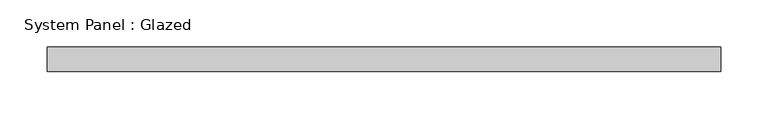
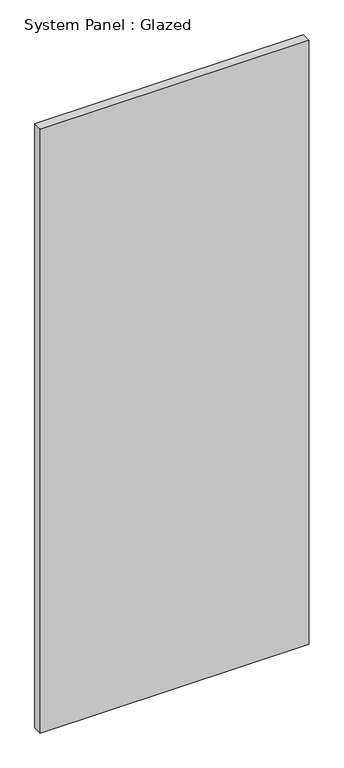
"""IFC4 building model written with IfcOpenShell, lengths in millimetres: plate geometry, System Panel : Glazed."""

from ifc_helpers import new_model, si_unit, origin, origin_with_axes, place, context, project, spatial, polyline, outline, extrude, source, transform, mapped, element, save


def system_panel_glazed_b47d4196(model_context):
    return source(origin(), model_context, "Body", "SweptSolid", [
        extrude(outline(polyline([(354.5271, 19.05), (-354.5271, 19.05), (-354.5271, 44.45), (354.5271, 44.45), (354.5271, 19.05)])), origin_with_axes(), (0.0, 0.0, 1.0), 1682.75),
    ])


if __name__ == "__main__":
    model = new_model("IFC4")
    model_context = context("Model", 3, world=origin())
    ifc_project = project(units=[si_unit("LENGTHUNIT", "METRE", prefix="MILLI")], contexts=[model_context])
    site = spatial("IfcSite", under=ifc_project)
    building = spatial("IfcBuilding", under=site)
    placement = place(None, origin())
    system_panel_glazed_shape = system_panel_glazed_b47d4196(model_context)
    element("IfcPlate", 1, ObjectType="System Panel : Glazed", at=placement, inside=building, context=model_context, shape_type="MappedRepresentation", body=[
        mapped(system_panel_glazed_shape, transform((0.0, 0.0, 0.0), x_axis=(1.0, 0.0, 0.0), y_axis=(0.0, 1.0, 0.0), z_axis=(0.0, 0.0, 1.0))),
    ])
    save(model, "model.ifc")

# Revit data of these elements
# Type "System Panel : Glazed"
#   Construction Type Id = "GSP4R"
#   Analytic Construction = "1/8 in Pilkington single glazing"
#   Visual Light Transmittance = 0.9
#   Solar Heat Gain Coefficient = 0.86
#   Heat Transfer Coefficient (U) = 1.18115 BTU/(h·ft²·°F)
#   Define Thermal Properties by = 1
# Element 1 (IfcPlate, "System Panel : Glazed")
#   Materials on its faces: "Glass"
# Materials
#   "Glass": class "Glass", colour RGB 0 128 192, transparency 0.75, Description = "Soda Lime Glass", Cost = 0
